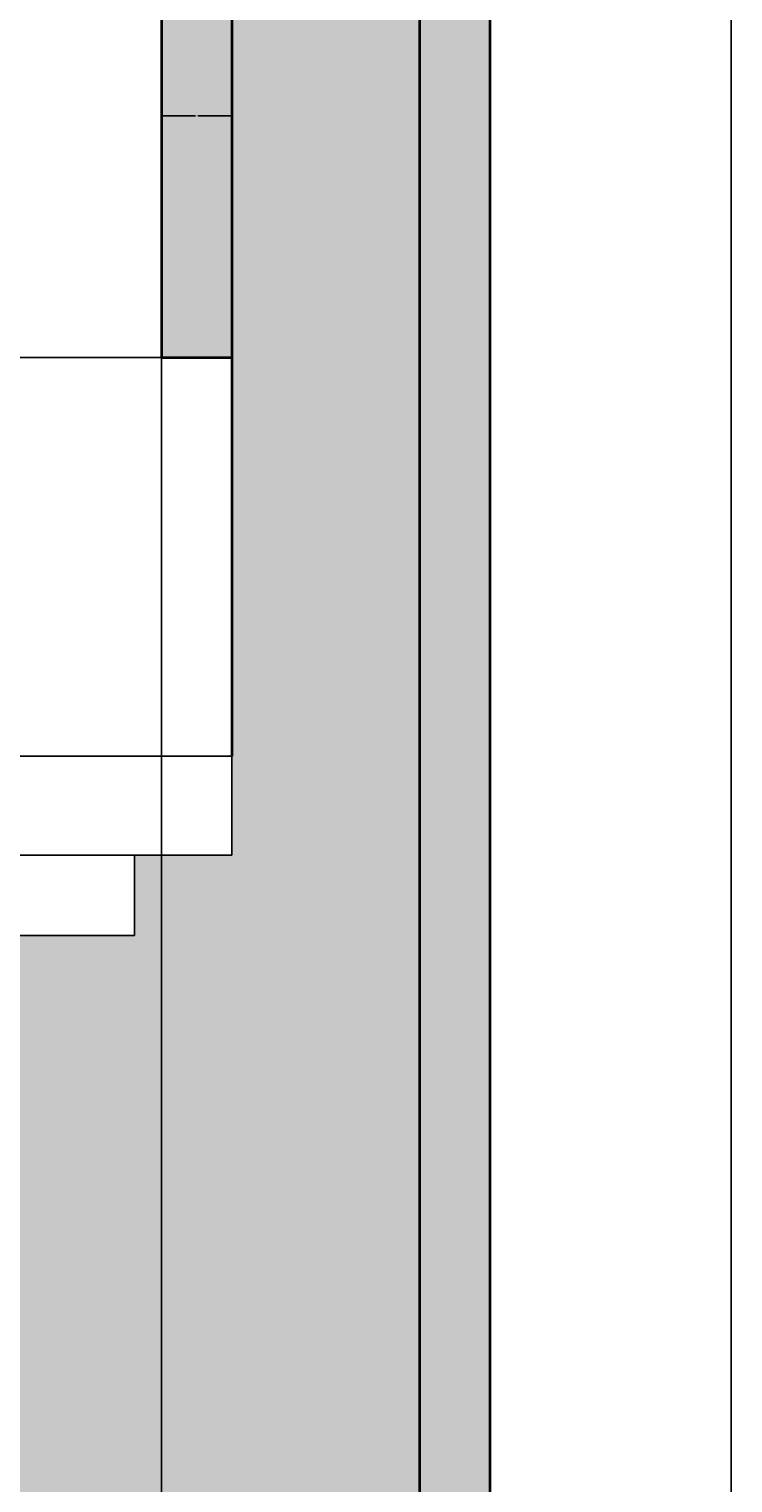
# Model space of a CAD drawing. Units: inches. Extents: x 2549 to 3108, y 1683 to 2362.
# Tile 5 of 30: x 3018 to 3108, y 1793 to 1979. Entities that reach past the tile are written whole.
import ezdxf

# ---------------------------------------------------------------- set-up
doc = ezdxf.new("R2010")
doc.units = ezdxf.units.IN
for name, color, linetype, lineweight in [('A-ANNO-DIMS', 2, 'Continuous', 18), ('A-FLOR', 7, 'Continuous', 25), ('A-FLOR-STRS', 7, 'Continuous', 25), ('A-WALL', 7, 'Continuous', 35), ('A-WALL-PATT', 89, 'Continuous', 13), ('C-PROP', 7, 'Continuous', 35)]:
    doc.layers.add(name, color=color, linetype=linetype, lineweight=lineweight)
doc.layers.add('C-PROP-PATT', color=252, linetype='Continuous', lineweight=13, true_color=0x939598)
doc.layers.add('C-PVMT-PATT', color=9, linetype='Continuous', lineweight=13, true_color=0xc7c8ca)
doc.styles.get("Standard").update_dxf_attribs({"font": 'arial.ttf'})
doc.dimstyles.get("Standard").update_dxf_attribs({"dimtxt": 0.18, "dimasz": 0.18, "dimexe": 0.18, "dimexo": 0.0625, "dimgap": 0.09, "dimtad": 0, "dimtih": 1, "dimtoh": 1, "dimdec": 4, "dimzin": 0, "dimdsep": 46, "dimtxsty": 'Standard', "dimcen": 0.09, "dimadec": 0, "dimazin": 0, "dimtfac": 1, "dimtdec": 4, "dimtofl": 0, "dimtmove": 0, "dimatfit": 3, "dimfxl": 1, "dimtolj": 1, "dimtzin": 0, "dimarcsym": 0})

# ---------------------------------------------------------------- blocks, each defined once
blk = doc.blocks.new('*D25')
at = {"layer": 'A-ANNO-DIMS', "color": 0, "lineweight": -2, "transparency": 16777216}
for p, q in [((3076.705166000002, 2314.523744000001), (3107.722666000003, 2314.523744000001)), ((3107.542666000004, 2314.343744000001), (3107.542666000004, 2014.705647137791)), ((3107.542666000004, 1714.703744000001), (3107.542666000004, 2014.341840862211)), ((3076.705166000002, 1714.523744000001), (3107.722666000003, 1714.523744000001))]:
    blk.add_line(p, q, dxfattribs=at)
at = {"layer": 'A-ANNO-DIMS', "color": 0, "transparency": 16777216}
for points in [[(3107.512666000003, 2314.343744000001), (3107.572666000004, 2314.343744000001), (3107.542666000004, 2314.523744000001)], [(3107.512666000003, 1714.703744000001), (3107.572666000004, 1714.703744000001), (3107.542666000004, 1714.523744000001)]]:
    blk.add_solid(points, dxfattribs=at)
at = {"layer": 'Defpoints', "color": 0, "transparency": 16777216}
for p in [(3076.642666000002, 2314.523744000001), (3107.542666000004, 2314.523744000001), (3076.642666000002, 1714.523744000001)]:
    blk.add_point(p, dxfattribs=at)
at = {"layer": 'A-ANNO-DIMS', "color": 0, "transparency": 16777216, "insert": (3107.542666000003, 2014.523743999999), "char_height": 0.18, "attachment_point": 5}
blk.add_mtext('\\A1;600', dxfattribs=at)
blk = doc.blocks.new('*D46')
at = {"layer": 'A-ANNO-DIMS', "color": 0, "lineweight": -2, "transparency": 16777216}
for p, q in [((2812.642666, 2140.461244), (2812.642666, 1683.443744)), ((3034.642666, 2134.461244), (3034.642666, 1683.443744)), ((2812.822666, 1683.623744), (2923.35320488131, 1683.623744)), ((3034.462666, 1683.623744), (2923.932127118691, 1683.623744))]:
    blk.add_line(p, q, dxfattribs=at)
at = {"layer": 'A-ANNO-DIMS', "color": 0, "transparency": 16777216}
for points in [[(2812.822666, 1683.653744), (2812.822666, 1683.593744), (2812.642666, 1683.623744)], [(3034.462666, 1683.653744), (3034.462666, 1683.593744), (3034.642666, 1683.623744)]]:
    blk.add_solid(points, dxfattribs=at)
at = {"layer": 'Defpoints', "color": 0, "transparency": 16777216}
for p in [(2812.642666, 2140.523744), (3034.642666, 2134.523744), (3034.642666, 1683.623744)]:
    blk.add_point(p, dxfattribs=at)
at = {"layer": 'A-ANNO-DIMS', "color": 0, "transparency": 16777216, "insert": (2923.642666000001, 1683.623744), "char_height": 0.18, "attachment_point": 5}
blk.add_mtext('\\A1;222', dxfattribs=at)
blk = doc.blocks.new('*D56')
at = {"layer": 'A-ANNO-DIMS', "color": 0, "lineweight": -2, "transparency": 16777216}
for p, q in [((3043.580166000001, 1936.523744000001), (2549.424763000002, 1936.523744000001)), ((2549.604763000002, 1936.343744000001), (2549.604763000002, 1911.205647137791)), ((2549.604763000002, 1885.703744000001), (2549.604763000002, 1910.841840862211)), ((3043.580166000001, 1885.523744000001), (2549.424763000002, 1885.523744000001))]:
    blk.add_line(p, q, dxfattribs=at)
at = {"layer": 'A-ANNO-DIMS', "color": 0, "transparency": 16777216}
for points in [[(2549.574763000002, 1936.343744000001), (2549.634763000002, 1936.343744000001), (2549.604763000002, 1936.523744000001)], [(2549.574763000002, 1885.703744000001), (2549.634763000002, 1885.703744000001), (2549.604763000002, 1885.523744000001)]]:
    blk.add_solid(points, dxfattribs=at)
at = {"layer": 'Defpoints', "color": 0, "transparency": 16777216}
for p in [(2549.604763000002, 1936.523744000001), (3043.642666000001, 1936.523744000001), (3043.642666000001, 1885.523744000001)]:
    blk.add_point(p, dxfattribs=at)
at = {"layer": 'A-ANNO-DIMS', "color": 0, "transparency": 16777216, "insert": (2549.604763000002, 1911.023743999999), "char_height": 0.18, "attachment_point": 5}
blk.add_mtext('\\A1;51', dxfattribs=at)
blk = doc.blocks.new('*D57')
at = {"layer": 'A-ANNO-DIMS', "color": 0, "lineweight": -2, "transparency": 16777216}
for p, q in [((2965.93514, 1936.586244), (2965.93514, 2362.322518)), ((2966.11514, 2362.142518), (2999.912081717599, 2362.142518)), ((3034.462666, 2362.142518), (3000.665724282401, 2362.142518)), ((3034.642666, 1936.586244), (3034.642666, 2362.322518))]:
    blk.add_line(p, q, dxfattribs=at)
at = {"layer": 'A-ANNO-DIMS', "color": 0, "transparency": 16777216}
for points in [[(2966.11514, 2362.172518), (2966.11514, 2362.112518), (2965.93514, 2362.142518)], [(3034.462666, 2362.172518), (3034.462666, 2362.112518), (3034.642666, 2362.142518)]]:
    blk.add_solid(points, dxfattribs=at)
at = {"layer": 'Defpoints', "color": 0, "transparency": 16777216}
for p in [(3034.642666, 2362.142518), (2965.93514, 1936.523744), (3034.642666, 1936.523744)]:
    blk.add_point(p, dxfattribs=at)
at = {"layer": 'A-ANNO-DIMS', "color": 0, "transparency": 16777216, "insert": (3000.288903, 2362.142518), "char_height": 0.18, "attachment_point": 5}
blk.add_mtext('\\A1;68.71', dxfattribs=at)
blk = doc.blocks.new('*D58')
at = {"layer": 'A-ANNO-DIMS', "color": 0, "lineweight": -2, "transparency": 16777216}
for p, q in [((3034.642666, 1936.586244), (3034.642666, 1967.603744)), ((3034.822666, 1967.423744), (3038.993484553888, 1967.423744)), ((3043.462666, 1967.423744), (3039.291847446112, 1967.423744)), ((3043.642666, 1936.586244), (3043.642666, 1967.603744))]:
    blk.add_line(p, q, dxfattribs=at)
at = {"layer": 'A-ANNO-DIMS', "color": 0, "transparency": 16777216}
for points in [[(3034.822666, 1967.453744), (3034.822666, 1967.393744), (3034.642666, 1967.423744)], [(3043.462666, 1967.453744), (3043.462666, 1967.393744), (3043.642666, 1967.423744)]]:
    blk.add_solid(points, dxfattribs=at)
at = {"layer": 'Defpoints', "color": 0, "transparency": 16777216}
for p in [(3043.642666, 1967.423744), (3034.642666, 1936.523744), (3043.642666, 1936.523744)]:
    blk.add_point(p, dxfattribs=at)
at = {"layer": 'A-ANNO-DIMS', "color": 0, "transparency": 16777216, "insert": (3039.142666, 1967.423744), "char_height": 0.18, "attachment_point": 5}
blk.add_mtext('\\A1;9', dxfattribs=at)

msp = doc.modelspace()

# ---------------------------------------------------------------- hatches: boundary and pattern name
at = {"layer": 'A-WALL-PATT'}
h = msp.add_hatch(color=256, dxfattribs=at)
h.dxf.hatch_style = 1
h.paths.add_polyline_path([(2638.642666391656, 2272.523744486262), (3034.642666391656, 2272.523744486262), (3034.642666391656, 1936.523744486262), (3043.642666391656, 1936.523744486262), (3043.642666391656, 2281.523744486262), (2629.642666391656, 2281.523744486262), (2629.642666391656, 2074.523744486262), (2812.642666391655, 2074.523744486262), (2812.642666391655, 2140.523744486262), (2785.717675498527, 2140.523744486262), (2785.717675498527, 2134.523744486262), (2806.642666391656, 2134.523744486262), (2806.642666391656, 2080.523744486262), (2638.642666391656, 2080.523744486262)])
h.paths.add_polyline_path([(2638.642666391656, 1972.523744486262), (2662.642666391656, 1972.523744486262), (2662.642666391656, 2041.055679691546), (2653.642666391655, 2041.055679691546), (2653.642666391656, 1978.523744486262), (2629.642666391656, 1978.523744486262), (2629.642666391656, 1795.523744486262), (2662.642666391656, 1795.523744486262), (2881.642666391656, 1795.523744486262), (2881.642666391656, 1936.523744486262), (2965.935139880862, 1936.523744486262), (2965.935139880862, 1974.543933838007), (2959.935139880861, 1974.543933838007), (2959.935139880861, 1945.523744486262), (2881.642666391656, 1945.523744486262), (2872.642666391655, 1945.523744486262), (2872.642666391655, 1804.523744486262), (2662.642666391656, 1804.523744486262), (2638.642666391656, 1804.523744486262)])
at = {"layer": 'C-PROP-PATT'}
h = msp.add_hatch(color=256, dxfattribs=at)
h.dxf.hatch_style = 1
h.paths.add_polyline_path([(3076.642666391656, 2314.523744486262), (2596.642666391656, 2314.523744486262), (2596.642666391656, 1714.523744486262), (2881.839988255281, 1714.523744486262), (2881.839988255281, 1723.523744486262), (2605.642666391656, 1723.523744486262), (2605.642666391656, 2305.523744486262), (3067.642666391656, 2305.523744486262), (3067.642666391656, 1723.523744486262), (3067.642666391656, 1714.523744486262), (3076.642666391656, 1714.523744486262)])
at = {"layer": 'C-PVMT-PATT'}
h = msp.add_hatch(color=256, dxfattribs=at)
h.dxf.hatch_style = 1
h.paths.add_polyline_path([(3067.642666391656, 2305.523744486262), (2605.642666391656, 2305.523744486262), (2605.642666391656, 2074.523744486262), (2629.642666391656, 2074.523744486262), (2629.642666391656, 2281.523744486262), (3043.642666391656, 2281.523744486262), (3043.642666391656, 1885.523744486263), (3043.642666391656, 1872.874514030248), (3031.167181590035, 1872.874514030248), (3031.167181590035, 1862.573058982011), (2995.805391311171, 1862.573058982011), (2995.805391311171, 1872.874514030248), (2983.175155144805, 1872.874514030248), (2983.175155144805, 1885.523744486262), (2881.642666391656, 1885.523744486263), (2881.642666391656, 1795.523744486262), (2751.09773888662, 1795.523744486262), (2751.09773888662, 1761.523744486262), (2786.157685455576, 1761.523744486262), (2786.157685455577, 1723.523744486262), (2881.839988255281, 1723.523744486262), (2881.839988255281, 1714.523744486262), (3067.642666391656, 1714.523744486262), (3067.642666391656, 1723.523744486262)])
edge = h.paths.add_edge_path(flags=16)
edge.add_ellipse((2949.440169726093, 1710.96831784248), major_axis=(-194.1013880556022, 3.100242e-10), ratio=0.8423038695451509, start_angle=-77.87403444762441, end_angle=-76.21947101041059, ccw=False)
edge.add_ellipse((2949.440169726089, 1715.215149574257), major_axis=(-189.1421864819335, 9.35831e-11), ratio=0.8423038695443681, start_angle=-79.7904610028283, end_angle=-77.55537270652758, ccw=False)
edge.add_ellipse((2899.927094610101, 2002.469218934773), major_axis=(155.4756451483881, 9.82606e-11), ratio=0.842303869543439, start_angle=-80.74343399283462, end_angle=-77.44506735589897)
edge.add_line((2928.591534983032, 1873.756406364807), (2932.388152113369, 1875.855825569603))
edge.add_line((2932.388152113369, 1875.855825569603), (2936.184769243706, 1873.756406364807))
edge.add_ellipse((2964.849209616638, 2002.469218934773), major_axis=(-155.4756451483861, 9.70869e-11), ratio=0.8423038695434499, start_angle=77.4450673558985, end_angle=80.74343399283416)
edge.add_ellipse((2915.336134500645, 1715.215149574254), major_axis=(189.1421864814668, 5.425418e-10), ratio=0.8423038695464061, start_angle=77.55537270639041, end_angle=79.79046100269102, ccw=False)
edge.add_ellipse((2915.336134500645, 1710.96831784248), major_axis=(-194.1013880561466, 2.794238e-10), ratio=0.8423038695428703, start_angle=256.2194710105847, end_angle=257.8740344477983, ccw=False)
edge.add_ellipse((2628.287132012546, 1850.261185811051), major_axis=(-327.2531525161749, 1.24457e-11), ratio=0.8423038695440036, start_angle=182.1799503136474, end_angle=183.6504275857012, ccw=False)
edge.add_ellipse((2955.563661936079, 1861.933375066942), major_axis=(-0.9167987925820851, 6.203e-13), ratio=0.8423038695438211, start_angle=180.0000000000388, end_angle=270.00000000003877, ccw=False)
edge.add_line((2956.480460728661, 1862.385732927092), (2956.480460728661, 1846.486613953928))
edge.add_ellipse((2955.563661936079, 1846.938971814078), major_axis=(-0.9167987925816303, 6.983e-13), ratio=0.8423038695442389, start_angle=90.0000000000436, end_angle=180.0000000000437, ccw=False)
edge.add_ellipse((-3607.060581297885, 1835.831972437108), major_axis=(-6562.624243233964, 2.000376e-10), ratio=0.8423038695434055, start_angle=179.6161332212093, end_angle=180.0902290885961, ccw=False)
edge.add_ellipse((2955.563661936079, 1791.092611498023), major_axis=(0.9167987925816303, 1.8053e-12), ratio=0.8423038695442389, start_angle=-1.127773430198431e-10, end_angle=89.99999999988711, ccw=False)
edge.add_line((2956.480460728661, 1791.544969358173), (2956.480460728661, 1775.645850385008))
edge.add_ellipse((2955.563661936079, 1776.098208245159), major_axis=(0.9167987925816303, 5.91e-14), ratio=0.8423038695442391, start_angle=269.9999999999963, end_angle=359.9999999999963, ccw=False)
edge.add_ellipse((-3607.060581297885, 1835.831972437108), major_axis=(-6562.624243233964, 2.000376e-10), ratio=0.8423038695434055, start_angle=179.3813568036826, end_angle=179.4717285281838, ccw=False)
edge.add_ellipse((2954.590723441648, 1763.876816393945), major_axis=(-1.375198188872997, 3.586e-13), ratio=0.8423038695436877, start_angle=179.3717627838213, end_angle=248.4647566010281, ccw=False)
edge.add_ellipse((-3607.518980694323, 1835.831972435604), major_axis=(-6564.040927375597, 4.0829067806e-06), ratio=0.8423038626957529, start_angle=179.3534459385899, end_angle=179.371762819423, ccw=False)
edge.add_ellipse((2952.682914207262, 1761.800246254478), major_axis=(3.250281735962, 3.921e-13), ratio=0.8423038695438826, start_angle=-89.99999999994031, end_angle=-0.6465540970884831, ccw=False)
edge.add_line((2952.682914207266, 1759.06252137117), (2912.093390019471, 1759.062521371171))
edge.add_ellipse((2912.093390019478, 1761.800246254481), major_axis=(3.250281735963338, 1.2841e-12), ratio=0.8423038695440954, start_angle=180.6465540970387, end_angle=269.99999999984414, ccw=False)
edge.add_ellipse((9472.295284948175, 1835.831972439052), major_axis=(-6564.040927413921, 8.323842912e-07), ratio=0.8423038709559154, start_angle=0.6282372235086768, end_angle=0.646554104341817, ccw=False)
edge.add_ellipse((2910.185580785089, 1763.876816393947), major_axis=(1.375198188873441, 9.687e-13), ratio=0.8423038695438604, start_angle=111.53524350397811, end_angle=180.6282372161342, ccw=False)
edge.add_ellipse((9471.836885542962, 1835.831972437208), major_axis=(-6562.624243252301, 3.836442e-10), ratio=0.8423038695462286, start_angle=0.5282714718206876, end_angle=0.6465540970643247, ccw=False)
edge.add_ellipse((2909.212642290659, 1776.098208245159), major_axis=(-0.9167987925820851, 6.203e-13), ratio=0.8423038695438211, start_angle=3.8824055081931874e-11, end_angle=90.00000000003882, ccw=False)
edge.add_line((2908.295843498077, 1775.645850385009), (2908.295843498077, 1791.544969358173))
edge.add_ellipse((2909.212642290659, 1791.092611498023), major_axis=(-0.9167987925820851, 4.868e-13), ratio=0.8423038695438213, start_angle=-89.99999999996948, end_angle=3.041122909053229e-11, ccw=False)
edge.add_ellipse((9471.836885542962, 1835.831972437208), major_axis=(-6562.624243252301, 3.836442e-10), ratio=0.8423038695462286, start_angle=-0.09022908858980827, end_angle=0.38386677879560693, ccw=False)
edge.add_ellipse((2909.212642290658, 1846.938971814078), major_axis=(-0.9167987925816306, 1.1661e-12), ratio=0.8423038695442389, start_angle=7.287326297955588e-11, end_angle=90.00000000007287, ccw=False)
edge.add_line((2908.295843498077, 1846.486613953928), (2908.295843498077, 1862.385732927092))
edge.add_ellipse((2909.212642290658, 1861.933375066942), major_axis=(0.9167987925816303, 1.1659e-12), ratio=0.8423038695442391, start_angle=89.99999999992713, end_angle=179.9999999999272, ccw=False)
edge.add_ellipse((3236.489172214191, 1850.261185811051), major_axis=(327.2531525161745, 3.33005e-11), ratio=0.8423038695444386, start_angle=176.3495724142951, end_angle=177.820049686349, ccw=False)
edge = h.paths.add_edge_path(flags=0)
edge.add_ellipse((2903.479330909537, 1857.335124490177), major_axis=(-34.79790434319148, 3.2087e-12), ratio=0.8423038695440206, start_angle=180.0000000000053, end_angle=209.4385695979841, ccw=False)
edge.add_line((2938.277235252728, 1857.335124490177), (2938.277235252728, 1855.879167118917))
edge.add_line((2938.277235252728, 1855.879167118917), (2939.463142736354, 1855.879167118917))
edge.add_line((2939.463142736354, 1855.879167118917), (2943.025124779096, 1853.39746861696))
edge.add_line((2943.025124779096, 1853.39746861696), (2943.025124779096, 1844.222223668088))
edge.add_ellipse((2940.651180015912, 1844.314306179491), major_axis=(0.2209272451118966, 3.927824345135514), ratio=0.6038335755719296, start_angle=106.3425919543001, end_angle=270.9979857249746, ccw=False)
edge.add_line((2938.277235252728, 1843.76085484809), (2938.277235252728, 1857.335124490177))
edge.add_ellipse((2903.479330909537, 1857.335124490177), major_axis=(-34.79790434319148, 3.2087e-12), ratio=0.8423038695440206, start_angle=180.0000000000052, end_angle=209.4385695979841)
edge.add_ellipse((2961.296973317201, 1857.335124490177), major_axis=(34.79790434319149, 1.2616e-12), ratio=0.8423038695439669, start_angle=150.5614304020187, end_angle=179.9999999999979)
edge.add_line((2926.49906897401, 1857.335124490177), (2926.49906897401, 1843.76085484809))
edge.add_ellipse((2924.125124210826, 1844.314306179491), major_axis=(-0.2209272451118966, 3.927824345135514), ratio=0.6038335755719296, start_angle=89.00201427502537, end_angle=253.65740804569998, ccw=False)
edge.add_line((2921.751179447642, 1844.222223668088), (2921.751179447642, 1853.39746861696))
edge.add_line((2921.751179447642, 1853.39746861696), (2925.313161490385, 1855.879167118917))
edge.add_line((2925.313161490385, 1855.879167118917), (2926.49906897401, 1855.879167118917))
edge.add_line((2926.49906897401, 1855.879167118917), (2926.49906897401, 1857.335124490177))
edge.add_ellipse((2961.296973317201, 1857.335124490177), major_axis=(34.79790434319149, 1.2616e-12), ratio=0.8423038695439669, start_angle=150.5614304020187, end_angle=179.999999999998, ccw=False)
edge = h.paths.add_edge_path(flags=0)
edge.add_ellipse((2929.050507673901, 1791.964048506909), major_axis=(50.66000311462998, 7.2698e-12), ratio=0.8423038695438956, start_angle=94.2774209630453, end_angle=111.8349537966997, ccw=False)
edge.add_line((2925.865275339109, 1834.550737322417), (2938.911028887629, 1834.550737322417))
edge.add_ellipse((2935.725796552836, 1791.96404850691), major_axis=(-50.6600031146233, 6.78e-13), ratio=0.8423038695439883, start_angle=248.16504620329118, end_angle=265.72257903694526, ccw=False)
edge.add_line((2951.925512935197, 1832.394679033669), (2950.571928129987, 1822.249450253823))
edge.add_ellipse((2934.122471365533, 1783.102276333124), major_axis=(49.30143828148681, 7.803e-13), ratio=0.8423038695439693, start_angle=67.20808512240917, end_angle=85.12993040286312)
edge.add_line((2937.651644899029, 1824.522535937876), (2927.12465932771, 1824.522535937876))
edge.add_ellipse((2930.653832861207, 1783.102276333115), major_axis=(-49.30143828149606, 1.1087e-12), ratio=0.8423038695440098, start_angle=-85.12993040286322, end_angle=-67.20808512241221)
edge.add_line((2914.204376096751, 1822.249450253823), (2912.850791291541, 1832.394679033669))
edge = h.paths.add_edge_path(flags=0)
edge.add_line((2910.133794844343, 1829.46512489105), (2912.643202843121, 1821.271117801794))
edge.add_ellipse((5203.77865552976, 1816.436683891122), major_axis=(-2291.142641748503, 9.8835e-11), ratio=0.8423038695495838, start_angle=-0.1208973690305054, end_angle=0.3640763488925343)
edge.add_line((2912.701209242743, 1801.878223466977), (2910.33046059899, 1792.569831244782))
edge.add_ellipse((9471.836885542954, 1835.831972437156), major_axis=(-6561.70744445971, 7.61654e-11), ratio=0.8423038695443023, start_angle=0.055594313499796044, end_angle=0.37776419391019544, ccw=False)
edge = h.paths.add_edge_path(flags=0)
edge.add_ellipse((-3607.060581316224, 1835.831972437187), major_axis=(6561.707444459722, 1.43187e-10), ratio=0.8423038695443235, start_angle=-0.37776419391110494, end_angle=-0.05559431350059185, ccw=False)
edge.add_line((2954.445843627751, 1792.569831244769), (2952.075094983995, 1801.878223466976))
edge.add_ellipse((660.9976486969767, 1816.436683891133), major_axis=(2291.142641748505, 5.276994e-10), ratio=0.842303869552366, start_angle=-0.3640763489035208, end_angle=0.1208973690194708)
edge.add_line((2952.133101383619, 1821.2711178018), (2954.642509382395, 1829.46512489105))
edge = h.paths.add_edge_path(flags=0)
edge.add_ellipse((2932.388152113369, 1865.19731394932), major_axis=(91.08099646002908, 7.134e-13), ratio=0.8423038695439837, start_angle=256.4018653097688, end_angle=283.5981346902299)
edge.add_line((2950.571928129987, 1790.023884530285), (2950.571928129987, 1778.362177885651))
edge.add_ellipse((2932.388152113369, 1853.535607304685), major_axis=(91.08099646002908, 7.134e-13), ratio=0.8423038695439837, start_angle=256.4018653097688, end_angle=283.5981346902299, ccw=False)
edge.add_line((2914.204376096751, 1778.362177885651), (2914.204376096751, 1790.023884530285))
edge = h.paths.add_edge_path(flags=0)
edge.add_line((2916.037973681915, 1773.858972345321), (2948.738330544823, 1773.85897234532))
edge.add_ellipse((2948.738330544823, 1772.31452600415), major_axis=(1.833597585163715, 1.1861e-12), ratio=0.8423038695440299, start_angle=-3.7118752516107634e-11, end_angle=89.999999999963, ccw=False)
edge.add_line((2950.571928129987, 1772.31452600415), (2950.571928129987, 1760.255799913308))
edge.add_line((2950.571928129987, 1760.255799913308), (2914.204376096751, 1760.255799913309))
edge.add_line((2914.204376096751, 1760.255799913309), (2914.204376096751, 1772.314526004151))
edge.add_ellipse((2916.037973681915, 1772.314526004151), major_axis=(1.833597585163716, 6.788e-13), ratio=0.84230386954403, start_angle=89.9999999999788, end_angle=179.9999999999788, ccw=False)
h.paths.add_polyline_path([(2629.642666391656, 1978.523744486262), (2605.642666391656, 1978.523744486262), (2605.642666391656, 1723.523744486262), (2629.642666391656, 1723.523744486262), (2629.642666391656, 1795.523744486262)], flags=17)
h.paths.add_polyline_path([(2800.524456569608, 1759.167447237475), (2853.743476964851, 1759.167447237475), (2853.743476964851, 1768.953962875417), (2800.524456569608, 1768.953962875417)], flags=24)
h.paths.add_polyline_path([(2972.461062245805, 1807.33049128039), (3015.394342810494, 1807.33049128039), (3015.394342810494, 1817.117006918332), (2972.461062245805, 1817.117006918332)], flags=24)

# ---------------------------------------------------------------- linework, layer by layer
at = {"layer": 'A-FLOR'}
msp.add_line((2881.642666391656, 1885.523744486263), (3043.642666391656, 1885.523744486262), dxfattribs=at)
at = {"layer": 'A-FLOR-STRS'}
for p, q in [((3043.642666391656, 1872.874514030248), (3043.642666391656, 1885.523744486262)), ((2983.175155144805, 1872.874514030248), (3043.642666391656, 1872.874514030248)), ((3031.167181590035, 1862.573058982011), (3031.167181590035, 1872.874514030248)), ((2995.805391311171, 1862.573058982011), (3031.167181590035, 1862.573058982011))]:
    msp.add_line(p, q, dxfattribs=at)
at = {"layer": 'A-WALL'}
for p, q in [((3043.642666391656, 2281.523744486262), (3043.642666391656, 1885.523744486263)), ((3034.642666391656, 2272.523744486262), (3034.642666391656, 1936.523744486262)), ((3034.642666391656, 1936.523744486262), (3043.642666391656, 1936.523744486262))]:
    msp.add_line(p, q, dxfattribs=at)
at = {"layer": 'C-PROP'}
msp.add_lwpolyline([(2596.642666391656, 2314.523744486262), (3076.642666391656, 2314.523744486262), (3076.642666391656, 1714.523744486262), (2596.642666391656, 1714.523744486262)], close=True, dxfattribs=at)
msp.add_lwpolyline([(2881.839988255281, 1723.523744486262), (2605.642666391656, 1723.523744486262), (2605.642666391656, 2305.523744486262), (3067.642666391656, 2305.523744486262), (3067.642666391656, 1723.523744486262)], dxfattribs=at)

# ---------------------------------------------------------------- dimensions: what is measured, and where the dimension line sits
at = {"layer": 'A-ANNO-DIMS'}
for base, p1, p2, override, picture, middle in [((3034.642666, 2362.142518), (2965.93514, 1936.523744), (3034.642666, 1936.523744), {"dimdec": 2, "dimlfac": 1, "dimrnd": 0, "dimzin": 0, "dimdsep": 46, "dimlunit": 2}, '*D57', (3000.288903, 2362.142518)), ((3034.642666, 1683.623744), (2812.642666, 2140.523744), (3034.642666, 2134.523744), {"dimdec": 0, "dimlfac": 1, "dimrnd": 0, "dimzin": 0, "dimdsep": 46, "dimlunit": 2}, '*D46', (2923.642666000001, 1683.623744)), ((3043.642666, 1967.423744), (3034.642666, 1936.523744), (3043.642666, 1936.523744), {"dimdec": 0, "dimlfac": 1, "dimrnd": 0, "dimzin": 0, "dimdsep": 46, "dimlunit": 2}, '*D58', (3039.142666, 1967.423744))]:
    dim = msp.add_linear_dim(base=base, p1=p1, p2=p2, dimstyle='Standard', override=override, dxfattribs=at)
    dim.commit()
    dim.dimension.update_dxf_attribs({"geometry": picture, "text_midpoint": middle})
for base, p1, p2, picture, middle in [((3107.542666000004, 2314.523744000001), (3076.642666000001, 1714.523744), (3076.642666000001, 2314.523744), '*D25', (3107.542666000003, 2014.523743999999)), ((2549.604763000002, 1936.523744000001), (3043.642666, 1885.523744), (3043.642666, 1936.523744), '*D56', (2549.604763000002, 1911.023743999999))]:
    dim = msp.add_linear_dim(base=base, p1=p1, p2=p2, angle=90, dimstyle='Standard', override={"dimdec": 0, "dimlfac": 1, "dimrnd": 0, "dimzin": 0, "dimdsep": 46, "dimlunit": 2}, dxfattribs=at)
    dim.commit()
    dim.dimension.update_dxf_attribs({"geometry": picture, "text_midpoint": middle})

doc.saveas('drawing.dxf')
